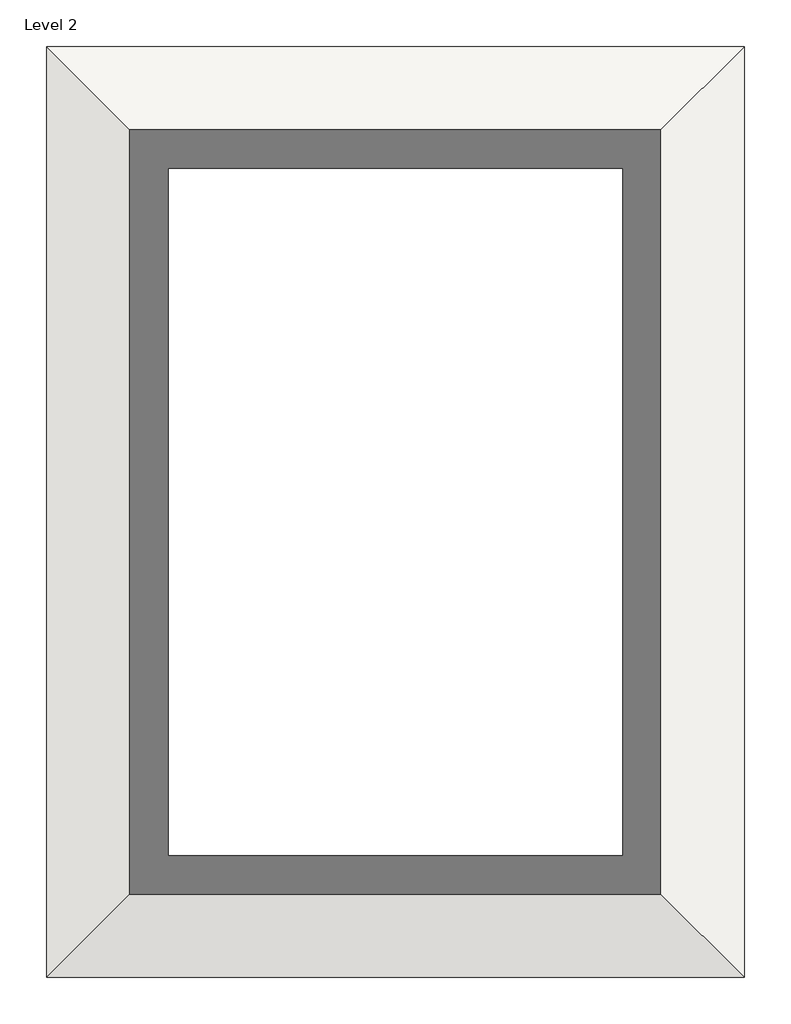
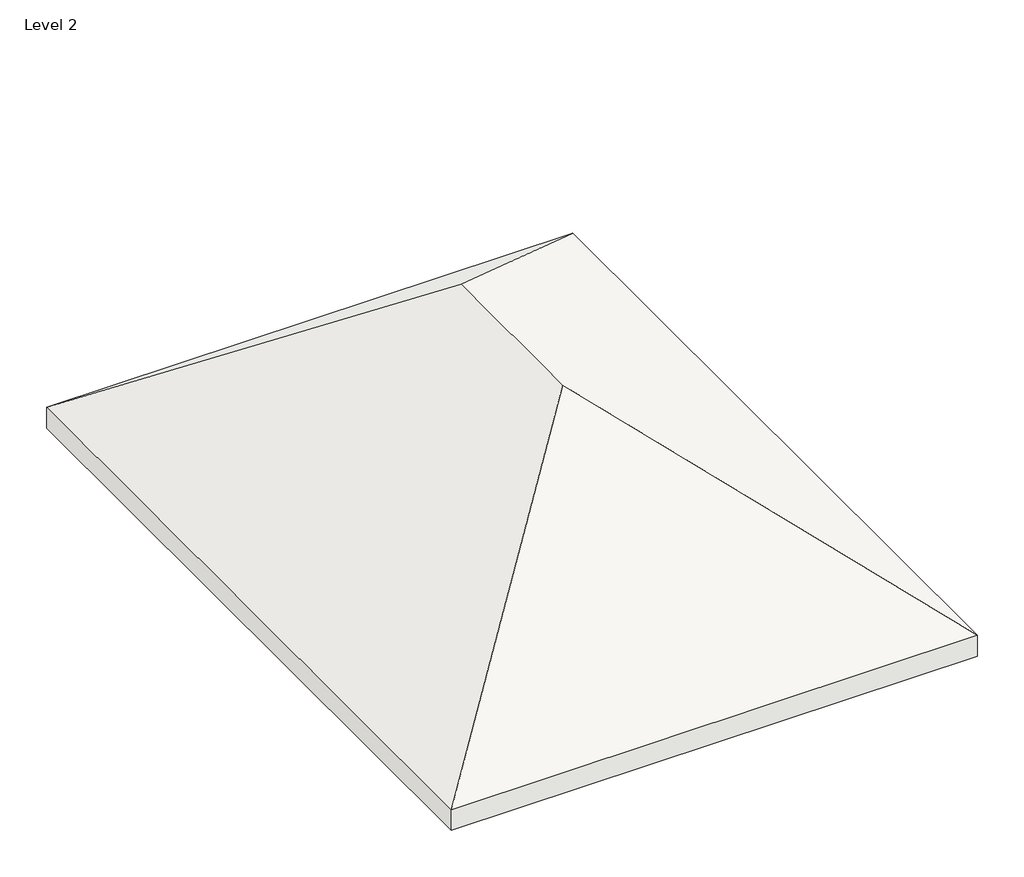
# One storey: 1 roof.
"""IFC4 building model written with IfcOpenShell, lengths in millimetres."""

from ifc_helpers import new_model, si_unit, origin, place, context, project, spatial, faceted_brep, element, save

model = new_model("IFC4")

# Units and contexts
model_context = context("Model", 3, world=origin())
ifc_project = project(units=[si_unit("LENGTHUNIT", "METRE", prefix="MILLI")], contexts=[model_context])

# Site, building, storey
site = spatial("IfcSite", under=ifc_project)
building = spatial("IfcBuilding", under=site)
storey = spatial("IfcBuildingStorey", under=building, Name="Level 2", Elevation=3048.0)

# Roof
placement = place(None, origin())
element("IfcRoof", 1, ObjectType="Generic - 12\"", at=placement, inside=storey, context=model_context, shape_type="Brep", body=[
    faceted_brep([(-6120.1806914, 4702.4715937, 6477.0), (-10692.1806914, 9274.4715937, 3048.0), (-1548.1806914, 9274.4715937, 3048.0), (-1548.1806914, -2917.5284063, 3048.0), (-6120.1806914, 1654.4715937, 6477.0), (-10692.1806914, -2917.5284063, 3048.0), (-10692.1806914, 9274.4715937, 3429.0), (-6120.1806914, 4702.4715937, 6858.0), (-1548.1806914, 9274.4715937, 3429.0), (-1548.1806914, -2917.5284063, 3429.0), (-6120.1806914, 1654.4715937, 6858.0), (-10692.1806914, -2917.5284063, 3429.0)], [[[0, 1, 2]], [[3, 4, 0, 2]], [[5, 4, 3]], [[1, 0, 4, 5]], [[6, 7, 8]], [[9, 8, 7, 10]], [[11, 9, 10]], [[6, 11, 10, 7]], [[5, 11, 6, 1]], [[3, 9, 11, 5]], [[2, 8, 9, 3]], [[1, 6, 8, 2]]]),
])

save(model, "model.ifc")

# Revit data of these elements
# Type "Generic - 12\""
#   Assembly Code = "B1020"
#   Layers, outside or top first: 1' - 0" no material (function 1)
# Element 1 (IfcRoof, "Generic - 12\"")
#   built-in parameter 1001705 = 22.5 (stored number, unit not read)
#   built-in parameter 1001710 = 33615
#   Phase Created = New Construction
#   Materials on its faces: "Default Roof"
# Materials
#   "Default Roof": colour RGB 88 101 114, transparency 0, Cost = 0
